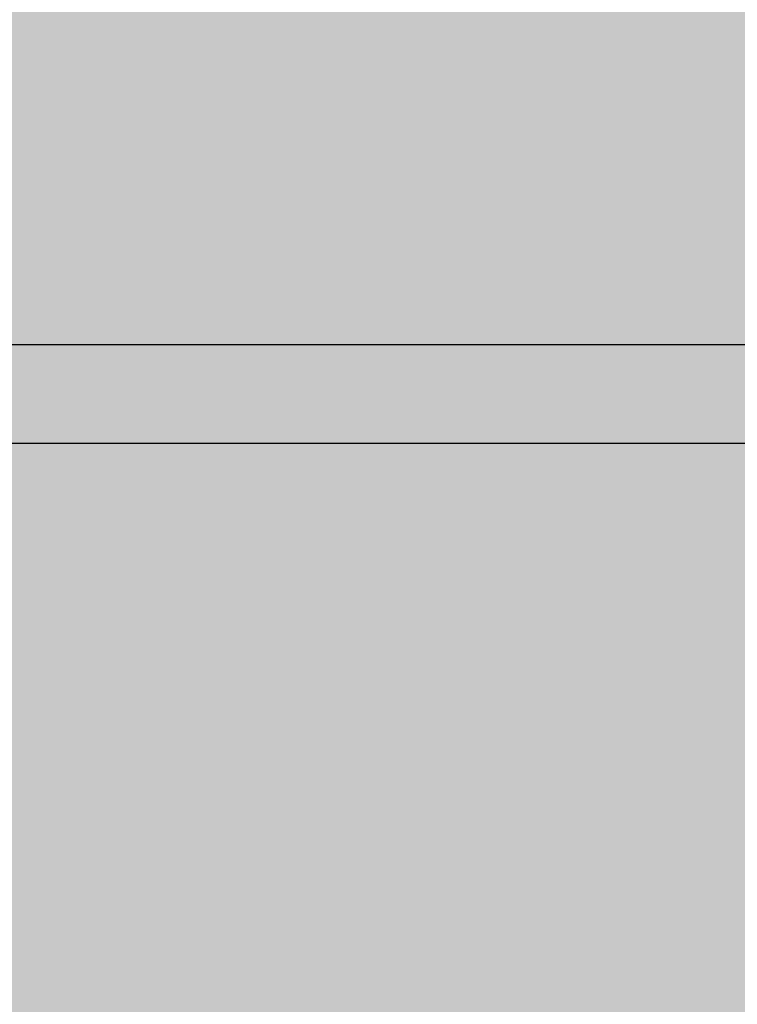
# Model space of a CAD drawing. Units: inches. Extents: x -12 to 334, y -10 to 186.
# Tile 58 of 77: x 127 to 145, y 111 to 136. Entities that reach past the tile are written whole.
import ezdxf
from ezdxf import colors
from ezdxf.entities.mleader import LeaderData, LeaderLine
from ezdxf.math import Vec2, Vec3

# ---------------------------------------------------------------- set-up
doc = ezdxf.new("R2010")
doc.units = ezdxf.units.IN
doc.header["$MEASUREMENT"] = 0
for name, color, linetype, lineweight in [('M-ANNO-TEXT', 3, 'Continuous', 25), ('M-DIMS', 2, 'Continuous', 18), ('M-EQPM-PATT', 8, 'Continuous', 18)]:
    doc.layers.add(name, color=color, linetype=linetype, lineweight=lineweight)
doc.styles.get("Standard").update_dxf_attribs({"font": 'arial.ttf'})
doc.dimstyles.get("Standard").update_dxf_attribs({"dimtxt": 0.18, "dimasz": 0.18, "dimexe": 0.18, "dimexo": 0.0625, "dimgap": 0.09, "dimtad": 0, "dimtih": 1, "dimtoh": 1, "dimdec": 4, "dimzin": 0, "dimdsep": 46, "dimtxsty": 'Standard', "dimcen": 0.09, "dimadec": 0, "dimazin": 0, "dimtfac": 1, "dimtdec": 4, "dimtofl": 0, "dimtmove": 0, "dimatfit": 3, "dimfxl": 1, "dimtolj": 1, "dimtzin": 0, "dimarcsym": 0})

# ---------------------------------------------------------------- blocks, each defined once
blk = doc.blocks.new('*D5')
at = {"layer": 'Defpoints', "color": 0, "transparency": 16777216}
for p in [(58.1, 127.708), (58.1, 125.208), (295.976, 125.208)]:
    blk.add_point(p, dxfattribs=at)
at = {"layer": 'M-DIMS', "color": 0, "lineweight": -2, "transparency": 16777216}
for p, q in [((58.163, 127.708), (296.156, 127.708)), ((295.976, 127.528), (295.976, 126.64)), ((295.976, 125.388), (295.976, 126.276)), ((58.163, 125.208), (296.156, 125.208))]:
    blk.add_line(p, q, dxfattribs=at)
at = {"layer": 'M-DIMS', "color": 0, "transparency": 16777216}
for points in [[(295.946, 127.528), (296.006, 127.528), (295.976, 127.708)], [(295.946, 125.388), (296.006, 125.388), (295.976, 125.208)]]:
    blk.add_solid(points, dxfattribs=at)
at = {"layer": 'M-DIMS', "color": 0, "transparency": 16777216, "insert": (295.976, 126.458), "char_height": 0.18, "attachment_point": 5}
blk.add_mtext('\\A1;2.5', dxfattribs=at)

msp = doc.modelspace()

# ---------------------------------------------------------------- hatches: boundary and pattern name
at = {"layer": 'M-EQPM-PATT', "transparency": 33554556}
h = msp.add_hatch(color=256, dxfattribs=at)
h.set_gradient(color1=(248, 206, 179), color2=(248, 206, 179), tint=1)
h.paths.add_polyline_path([(179.7818, 136.8871), (126.9567, 136.8871), (106.1771, 100.8958), (171.5458, 100.8958)])
h.paths.add_polyline_path([(268.3808, 136.9435), (214.0166, 136.9435), (214.0166, 154.8345), (196.3421, 154.8345), (196.3421, 136.8871), (179.7818, 136.8871), (171.5458, 100.8958), (231.7758, 100.8958, -0.4142136), (251.9801, 80.6915), (279.7263, 80.6915, 0.1631825)])

# ---------------------------------------------------------------- dimensions: what is measured, and where the dimension line sits
at = {"layer": 'M-DIMS'}
dim = msp.add_linear_dim(base=(295.9756, 125.2078), p1=(58.1002, 127.7078), p2=(58.1002, 125.2078), angle=90, dimstyle='Standard', override={"dimdec": 1, "dimlfac": 1, "dimrnd": 0, "dimzin": 0, "dimdsep": 46, "dimlunit": 2}, dxfattribs=at)
dim.commit()
dim.dimension.update_dxf_attribs({"geometry": '*D5', "text_midpoint": (295.9756, 126.4578)})

# ---------------------------------------------------------------- leaders
at = {"layer": 'M-ANNO-TEXT'}
ml = msp.add_multileader_mtext('Standard', dxfattribs=at)
ml.set_content('Tube supports', color=256)
ml.set_leader_properties()
ml.build(insert=Vec2(0, 0))
ml.multileader.update_dxf_attribs({"dogleg_length": 0.36, "arrow_head_size": 0.7})
ctx = ml.context
ctx.base_point, ctx.arrow_head_size, ctx.landing_gap_size, ctx.plane_origin = Vec3(129.4363, 148.4609), 0.7, 0.09, Vec3(117.375, 151.6517)
ctx.text_align_type = 2
notes = []
notes.append((ctx, [(1, (1, 1, 0), (182.4302, 148.4609), (-1, 0), 17.4388, [(0, [(170.9079, 98.1081)], 0, [])])]))
ctx.mtext.insert, ctx.mtext.alignment, ctx.mtext.flow_direction = Vec3(164.9015, 151.0162), 3, 5
for ctx, leaders in notes:
    for number, flags, end, landing, length, lines in leaders:
        leader = LeaderData()
        leader.index, (leader.has_last_leader_line, leader.has_dogleg_vector, leader.attachment_direction) = number, flags
        leader.last_leader_point, leader.dogleg_vector, leader.dogleg_length = Vec3(end), Vec3(landing), length
        for number, points, colour, breaks in lines:
            line = LeaderLine()
            line.index, line.vertices, line.color, line.breaks = number, Vec3.list(points), colors.encode_raw_color(colour), breaks
            leader.lines.append(line)
        ctx.leaders.append(leader)

doc.saveas('drawing.dxf')
